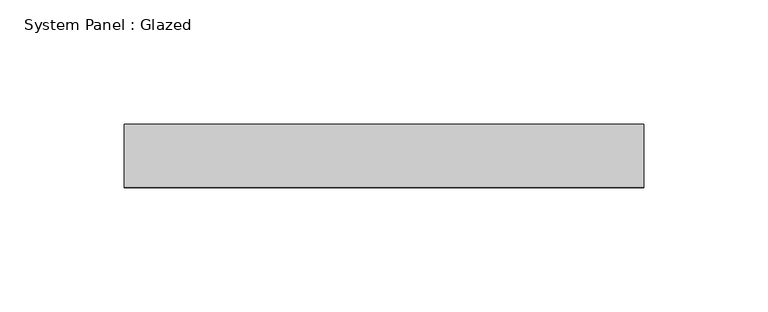
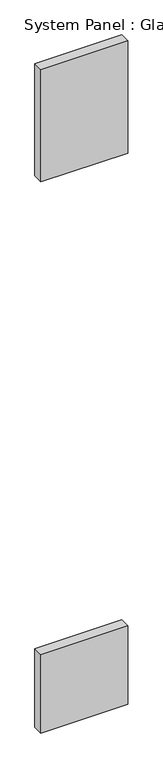
"""IFC4 building model written with IfcOpenShell, lengths in millimetres: plate geometry, System Panel : Glazed."""

from ifc_helpers import new_model, si_unit, frame, origin, origin_with_axes, place, context, project, spatial, polyline, outline, extrude, source, transform, mapped, element, save


def system_panel_glazed_026653f5(model_context):
    return source(origin(), model_context, "Body", "SweptSolid", [
        extrude(outline(polyline([(104.775, 19.05), (-104.775, 19.05), (-104.775, 44.45), (104.775, 44.45), (104.775, 19.05)])), origin_with_axes(), (0.0, 0.0, 1.0), 199.39),
        extrude(outline(polyline([(104.775, 19.05), (-104.775, 19.05), (-104.775, 44.45), (104.775, 44.45), (104.775, 19.05)])), frame((0.0, 0.0, 1403.35), z_axis=(0.0, 0.0, 1.0), x_axis=(1.0, 0.0, 0.0)), (0.0, 0.0, 1.0), 285.75),
    ])


if __name__ == "__main__":
    model = new_model("IFC4")
    model_context = context("Model", 3, world=origin())
    ifc_project = project(units=[si_unit("LENGTHUNIT", "METRE", prefix="MILLI")], contexts=[model_context])
    site = spatial("IfcSite", under=ifc_project)
    building = spatial("IfcBuilding", under=site)
    placement = place(None, origin())
    system_panel_glazed_shape = system_panel_glazed_026653f5(model_context)
    element("IfcPlate", 1, ObjectType="System Panel : Glazed", at=placement, inside=building, context=model_context, shape_type="MappedRepresentation", body=[
        mapped(system_panel_glazed_shape, transform((0.0, 0.0, 0.0), x_axis=(1.0, 0.0, 0.0), y_axis=(0.0, 1.0, 0.0), z_axis=(0.0, 0.0, 1.0))),
    ])
    save(model, "model.ifc")

# Revit data of these elements
# Type "System Panel : Glazed"
#   Construction Type Id = "GSP4R"
#   Analytic Construction = "1/8 in Pilkington single glazing"
#   Visual Light Transmittance = 0.9
#   Solar Heat Gain Coefficient = 0.86
#   Heat Transfer Coefficient (U) = 1.18115 BTU/(h·ft²·°F)
#   Define Thermal Properties by = 1
# Element 1 (IfcPlate, "System Panel : Glazed")
#   Materials on its faces: "Glass"
# Materials
#   "Glass": class "Glass", colour RGB 0 128 192, transparency 0.75, Description = "Soda Lime Glass", Cost = 0
